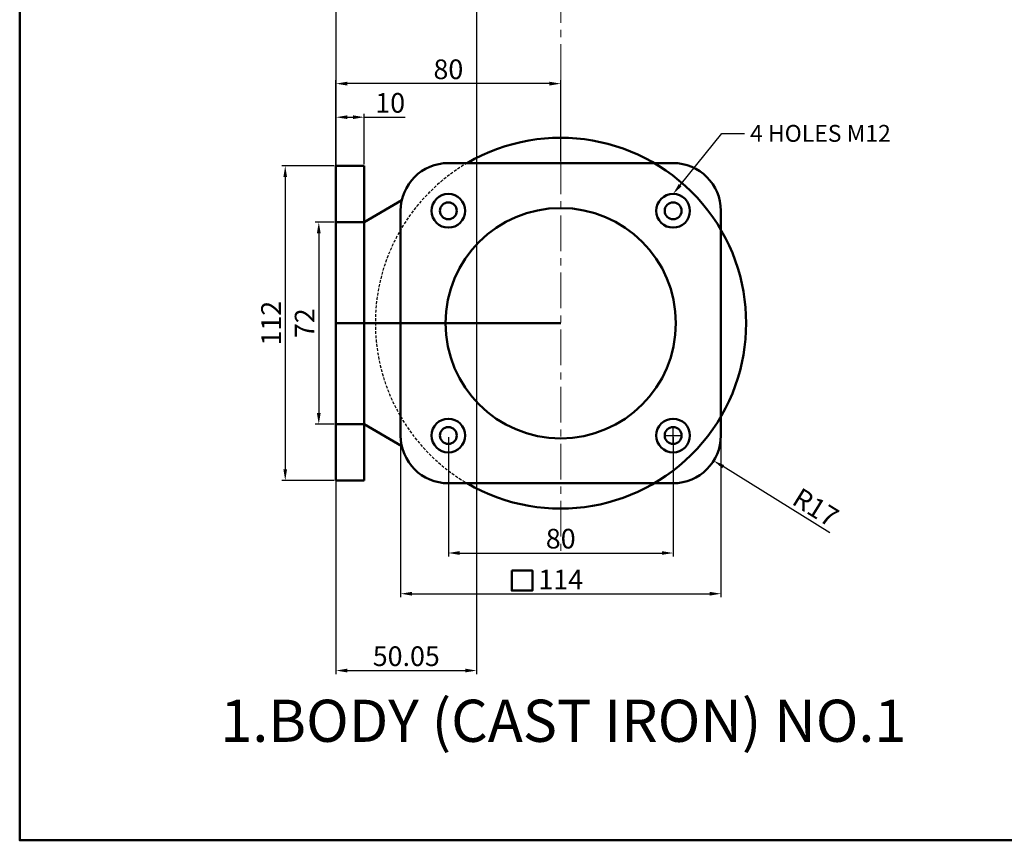
# Model space of a CAD drawing. Units: millimetres. Extents: x 49 to 1001, y -335 to 311.
# Tile 1 of 4: x 49 to 399, y -335 to -43. Entities that reach past the tile are written whole.
import ezdxf
from ezdxf import colors
from ezdxf.entities.mleader import LeaderData, LeaderLine
from ezdxf.math import Vec2, Vec3

# ---------------------------------------------------------------- set-up
doc = ezdxf.new("R2010")
doc.units = ezdxf.units.MM
doc.header["$LTSCALE"] = 0.4
doc.linetypes.add('CENTER', pattern=[50.8, 31.75, -6.35, 6.35, -6.35])
doc.linetypes.add('HIDDEN', pattern=[9.525, 6.35, -3.175])
for name, color, linetype, lineweight in [('M-CNTR', 1, 'CENTER', 18), ('M-DIMS', 2, 'Continuous', 25), ('M-HIDN', 6, 'HIDDEN', 25), ('M-OUTL', 7, 'Continuous', 50), ('M-TEXT', 3, 'Continuous', 25)]:
    doc.layers.add(name, color=color, linetype=linetype, lineweight=lineweight)
doc.styles.get("Standard").update_dxf_attribs({"font": 'arial.ttf'})
doc.dimstyles.new('ISO-25', dxfattribs={"dimtxt": 7, "dimasz": 4, "dimexe": 1.25, "dimexo": 0.625, "dimtad": 1, "dimtxsty": 'Standard', "dimcen": 2.5, "dimadec": 0, "dimazin": 0, "dimtfac": 1, "dimtofl": 0, "dimtmove": 0, "dimatfit": 3, "dimfxl": 1, "dimarcsym": 0})

# ---------------------------------------------------------------- blocks, each defined once
blk = doc.blocks.new('*D17')
at = {"layer": 'Defpoints', "color": 0, "ltscale": 0.4, "transparency": 16777216}
for p in [(171.24, -77.64), (161.24, -94.96), (171.24, -94.96)]:
    blk.add_point(p, dxfattribs=at)
at = {"layer": 'M-DIMS', "color": 0, "lineweight": -2, "ltscale": 0.4, "transparency": 16777216}
for p, q in [((161.24, -94.34), (161.24, -76.39)), ((171.24, -94.34), (171.24, -76.39)), ((165.24, -77.64), (167.24, -77.64)), ((171.24, -77.64), (185.83, -77.64))]:
    blk.add_line(p, q, dxfattribs=at)
at = {"layer": 'M-DIMS', "color": 0, "ltscale": 0.4, "transparency": 16777216}
for points in [[(165.24, -76.97), (165.24, -78.3), (161.24, -77.64)], [(167.24, -76.97), (167.24, -78.3), (171.24, -77.64)]]:
    blk.add_solid(points, dxfattribs=at)
at = {"layer": 'M-DIMS', "color": 0, "ltscale": 0.4, "transparency": 16777216, "insert": (180.53, -73.44), "char_height": 7, "attachment_point": 5}
blk.add_mtext('10', dxfattribs=at)
blk = doc.blocks.new('*D18')
at = {"layer": 'Defpoints', "color": 0, "ltscale": 0.4, "transparency": 16777216}
for p in [(161.24, -94.96), (143.17, -206.96), (161.24, -206.96)]:
    blk.add_point(p, dxfattribs=at)
at = {"layer": 'M-DIMS', "color": 0, "lineweight": -2, "ltscale": 0.4, "transparency": 16777216}
for p, q in [((160.61, -94.96), (141.92, -94.96)), ((143.17, -98.96), (143.17, -202.96)), ((160.61, -206.96), (141.92, -206.96))]:
    blk.add_line(p, q, dxfattribs=at)
at = {"layer": 'M-DIMS', "color": 0, "ltscale": 0.4, "transparency": 16777216}
for points in [[(142.5, -98.96), (143.83, -98.96), (143.17, -94.96)], [(142.5, -202.96), (143.83, -202.96), (143.17, -206.96)]]:
    blk.add_solid(points, dxfattribs=at)
at = {"layer": 'M-DIMS', "color": 0, "ltscale": 0.4, "transparency": 16777216, "insert": (139.03, -150.96), "char_height": 7, "attachment_point": 5, "rotation": 90}
blk.add_mtext('112', dxfattribs=at)
blk = doc.blocks.new('*D19')
at = {"layer": 'Defpoints', "color": 0, "ltscale": 0.4, "transparency": 16777216}
for p in [(161.24, -114.96), (155.12, -186.96), (161.24, -186.96)]:
    blk.add_point(p, dxfattribs=at)
at = {"layer": 'M-DIMS', "color": 0, "lineweight": -2, "ltscale": 0.4, "transparency": 16777216}
for p, q in [((160.61, -114.96), (153.87, -114.96)), ((155.12, -118.96), (155.12, -182.96)), ((160.61, -186.96), (153.87, -186.96))]:
    blk.add_line(p, q, dxfattribs=at)
at = {"layer": 'M-DIMS', "color": 0, "ltscale": 0.4, "transparency": 16777216}
for points in [[(154.45, -118.96), (155.78, -118.96), (155.12, -114.96)], [(154.45, -182.96), (155.78, -182.96), (155.12, -186.96)]]:
    blk.add_solid(points, dxfattribs=at)
at = {"layer": 'M-DIMS', "color": 0, "ltscale": 0.4, "transparency": 16777216, "insert": (150.98, -150.96), "char_height": 7, "attachment_point": 5, "rotation": 90}
blk.add_mtext('72', dxfattribs=at)
blk = doc.blocks.new('*D20')
at = {"layer": 'Defpoints', "color": 0, "ltscale": 0.4, "transparency": 16777216}
for p in [(161.24, -65.69), (241.24, -93.96), (161.24, -114.96)]:
    blk.add_point(p, dxfattribs=at)
at = {"layer": 'M-DIMS', "color": 0, "lineweight": -2, "ltscale": 0.4, "transparency": 16777216}
for p, q in [((161.24, -114.34), (161.24, -64.44)), ((237.24, -65.69), (165.24, -65.69)), ((241.24, -93.34), (241.24, -64.44))]:
    blk.add_line(p, q, dxfattribs=at)
at = {"layer": 'M-DIMS', "color": 0, "ltscale": 0.4, "transparency": 16777216}
for points in [[(165.24, -65.02), (165.24, -66.36), (161.24, -65.69)], [(237.24, -65.02), (237.24, -66.36), (241.24, -65.69)]]:
    blk.add_solid(points, dxfattribs=at)
at = {"layer": 'M-DIMS', "color": 0, "ltscale": 0.4, "transparency": 16777216, "insert": (201.24, -61.49), "char_height": 7, "attachment_point": 5}
blk.add_mtext('80', dxfattribs=at)
blk = doc.blocks.new('*D21')
at = {"layer": 'Defpoints', "color": 0, "ltscale": 0.4, "transparency": 16777216}
for p in [(298.24, -173.69), (184.24, -178.8), (298.24, -247.27)]:
    blk.add_point(p, dxfattribs=at)
at = {"layer": 'M-DIMS', "color": 0, "lineweight": -2, "ltscale": 0.4, "transparency": 16777216}
for p, q in [((298.24, -174.31), (298.24, -248.52)), ((184.24, -179.42), (184.24, -248.52)), ((188.24, -247.27), (294.24, -247.27))]:
    blk.add_line(p, q, dxfattribs=at)
at = {"layer": 'M-DIMS', "color": 0, "ltscale": 0.4, "transparency": 16777216}
for points in [[(188.24, -246.6), (188.24, -247.94), (184.24, -247.27)], [(294.24, -246.6), (294.24, -247.94), (298.24, -247.27)]]:
    blk.add_solid(points, dxfattribs=at)
at = {"layer": 'M-DIMS', "color": 0, "ltscale": 0.4, "transparency": 16777216, "insert": (241.24, -243.13), "char_height": 7, "attachment_point": 5}
blk.add_mtext('114', dxfattribs=at)
blk = doc.blocks.new('*D22')
at = {"layer": 'Defpoints', "color": 0, "ltscale": 0.4, "transparency": 16777216}
for p in [(201.24, -190.96), (281.24, -190.96), (281.24, -232.78)]:
    blk.add_point(p, dxfattribs=at)
at = {"layer": 'M-DIMS', "color": 0, "lineweight": -2, "ltscale": 0.4, "transparency": 16777216}
for p, q in [((201.24, -191.59), (201.24, -234.03)), ((281.24, -191.59), (281.24, -234.03)), ((205.24, -232.78), (277.24, -232.78))]:
    blk.add_line(p, q, dxfattribs=at)
at = {"layer": 'M-DIMS', "color": 0, "ltscale": 0.4, "transparency": 16777216}
for points in [[(205.24, -232.11), (205.24, -233.44), (201.24, -232.78)], [(277.24, -232.11), (277.24, -233.44), (281.24, -232.78)]]:
    blk.add_solid(points, dxfattribs=at)
at = {"layer": 'M-DIMS', "color": 0, "ltscale": 0.4, "transparency": 16777216, "insert": (241.24, -228.58), "char_height": 7, "attachment_point": 5}
blk.add_mtext('80', dxfattribs=at)
blk = doc.blocks.new('*D23')
at = {"layer": 'Defpoints', "color": 0, "ltscale": 0.4, "transparency": 16777216}
for p in [(281.24, -190.96), (295.68, -199.93)]:
    blk.add_point(p, dxfattribs=at)
at = {"layer": 'M-DIMS', "color": 0, "lineweight": -2, "ltscale": 0.4, "transparency": 16777216}
for p, q in [((281.24, -193.46), (281.24, -188.46)), ((278.74, -190.96), (283.74, -190.96)), ((336.99, -225.58), (299.08, -202.04))]:
    blk.add_line(p, q, dxfattribs=at)
at = {"layer": 'M-DIMS', "color": 0, "ltscale": 0.4, "transparency": 16777216}
blk.add_solid([(299.43, -201.47), (298.73, -202.61), (295.68, -199.93)], dxfattribs=at)
at = {"layer": 'M-DIMS', "color": 0, "ltscale": 0.4, "transparency": 16777216, "insert": (331.53, -217.32), "char_height": 7, "attachment_point": 5, "rotation": 328.1606}
blk.add_mtext('R17', dxfattribs=at)
blk = doc.blocks.new('BOLT-HOLE-12')
at = {"ltscale": 0.4}
for radius in [6, 3]:
    blk.add_circle((6, 6), radius, dxfattribs=at)
blk = doc.blocks.new('*D58')
at = {"layer": 'Defpoints', "color": 0, "ltscale": 0.4, "transparency": 16777216}
for p in [(211.28, 81.71), (161.24, 58.7), (211.28, -274.62)]:
    blk.add_point(p, dxfattribs=at)
at = {"layer": 'M-DIMS', "color": 0, "lineweight": -2, "ltscale": 0.4, "transparency": 16777216}
for p, q in [((211.28, 81.09), (211.28, -275.87)), ((161.24, 58.08), (161.24, -275.87)), ((165.24, -274.62), (207.28, -274.62))]:
    blk.add_line(p, q, dxfattribs=at)
at = {"layer": 'M-DIMS', "color": 0, "ltscale": 0.4, "transparency": 16777216}
for points in [[(165.24, -273.95), (165.24, -275.28), (161.24, -274.62)], [(207.28, -273.95), (207.28, -275.28), (211.28, -274.62)]]:
    blk.add_solid(points, dxfattribs=at)
at = {"layer": 'M-DIMS', "color": 0, "ltscale": 0.4, "transparency": 16777216, "insert": (186.26, -270.42), "char_height": 7, "attachment_point": 5}
blk.add_mtext('50.05', dxfattribs=at)

msp = doc.modelspace()

# ---------------------------------------------------------------- linework, layer by layer
at = {"layer": 'M-CNTR'}
msp.add_line((241.2373, 232.8267), (241.2373, -233.1822), dxfattribs=at)
at = {"layer": 'M-HIDN', "ltscale": 0.4}
msp.add_arc((241.2373, -150.9613), 66, 120.272641, 239.727359, dxfattribs=at)
at = {"layer": 'M-OUTL', "ltscale": 0.4}
for p, q in [((161.2373, -150.9613), (161.2373, -94.9613)), ((161.2373, -94.9613), (171.2373, -94.9613)), ((171.2373, -94.9613), (171.2373, -206.9613)), ((171.2373, -114.9613), (184.6554, -107.2144)), ((171.2373, -114.9613), (161.2373, -114.9613)), ((241.2373, -150.9613), (161.2373, -150.9613)), ((161.2373, -206.9613), (161.2373, -150.9613)), ((171.2373, -186.9613), (161.2373, -186.9613)), ((171.2373, -186.9613), (184.6554, -194.7082)), ((171.2373, -206.9613), (161.2373, -206.9613))]:
    msp.add_line(p, q, dxfattribs=at)
for points in [[(48.6466, 311.3462), (1001.3348, 311.3462), (1001.3348, -335.0483), (48.6466, -335.0483)], [(223.8267, -239.0323), (231.1417, -239.0323), (231.1417, -246.1666), (223.8267, -246.1666)]]:
    msp.add_lwpolyline(points, close=True, dxfattribs=at)
msp.add_lwpolyline([(201.2373, -93.9613), (281.2373, -93.9613, -0.41421356), (298.2373, -110.9613), (298.2373, -190.9613, -0.41421356), (281.2373, -207.9613), (201.2373, -207.9613, -0.41421356), (184.2373, -190.9613), (184.2373, -110.9613, -0.41421356)], format="xyb", close=True, dxfattribs=at)
msp.add_circle((241.2373, -150.9613), 41, dxfattribs=at)
msp.add_arc((241.2373, -150.9613), 66, 239.727359, 120.272641, dxfattribs=at)

# ---------------------------------------------------------------- block references
at = {"layer": 'M-OUTL'}
for p in [(195.237, -116.961), (275.237, -116.961), (195.237, -196.961), (275.237, -196.961)]:
    msp.add_blockref('BOLT-HOLE-12', p, dxfattribs=at)

# ---------------------------------------------------------------- texts
at = {"layer": 'M-TEXT', "ltscale": 0.4, "insert": (120.105, -284.9979), "char_height": 15, "attachment_point": 1}
msp.add_mtext_dynamic_manual_height_columns('1.BODY (CAST IRON) NO.1', width=263.462389, gutter_width=12.5, heights=[0], dxfattribs=at)

# ---------------------------------------------------------------- dimensions: what is measured, and where the dimension line sits
at = {"layer": 'M-DIMS', "ltscale": 0.4}
for base, p1, p2, override, picture, middle in [((211.2829, -274.6166), (161.2373, 58.7021), (211.2829, 81.7143), {"dimdec": 2, "dimlfac": 1, "dimrnd": 0, "dimzin": 0, "dimdsep": 46, "dimlunit": 2}, '*D58', (186.2601, -270.4176)), ((161.2373, -65.6885), (241.2373, -93.9613), (161.2373, -114.9613), {"dimclrd": 0, "dimclre": 0, "dimclrt": 0}, '*D20', (201.2373, -61.4895)), ((171.2373, -77.6381), (161.2373, -94.9613), (171.2373, -94.9613), {"dimclrd": 0, "dimclre": 0, "dimclrt": 0}, '*D17', (180.5346, -73.439)), ((298.2373, -247.2713), (184.2373, -178.7991), (298.2373, -173.6859), {"dimclrd": 0, "dimclre": 0, "dimclrt": 0}, '*D21', (241.2373, -243.132)), ((281.2373, -232.777), (201.2373, -190.9613), (281.2373, -190.9613), {"dimclrd": 0, "dimclre": 0, "dimclrt": 0}, '*D22', (241.2373, -228.5779))]:
    dim = msp.add_linear_dim(base=base, p1=p1, p2=p2, dimstyle='ISO-25', override=override, dxfattribs=at)
    dim.commit()
    dim.dimension.update_dxf_attribs({"geometry": picture, "text_midpoint": middle})
for base, p1, p2, picture, middle in [((143.1676, -206.9613), (161.2373, -94.9613), (161.2373, -206.9613), '*D18', (139.0282, -150.9613)), ((155.1167, -186.9613), (161.2373, -114.9613), (161.2373, -186.9613), '*D19', (150.9774, -150.9613))]:
    dim = msp.add_linear_dim(base=base, p1=p1, p2=p2, angle=90, dimstyle='ISO-25', override={"dimclrd": 0, "dimclre": 0, "dimclrt": 0}, dxfattribs=at)
    dim.commit()
    dim.dimension.update_dxf_attribs({"geometry": picture, "text_midpoint": middle})
dim = msp.add_radius_dim(center=(281.2373, -190.9613), mpoint=(295.6793, -199.9295), dimstyle='ISO-25', override={"dimclrd": 0, "dimclre": 0, "dimclrt": 0}, dxfattribs=at)
dim.commit()
dim.dimension.update_dxf_attribs({"geometry": '*D23', "text_midpoint": (329.351, -220.8389), "dimtype": 164})

# ---------------------------------------------------------------- leaders
ml = msp.add_multileader_mtext('Standard', dxfattribs=at)
ml.set_content('4 HOLES M12', color=256)
ml.set_leader_properties()
ml.build(insert=Vec2(0, 0))
ctx = ml.context
ctx.base_point, ctx.char_height, ctx.plane_origin = Vec3(306.621, -83.4432), 6, Vec3(281.2373, -104.9613)
notes = []
notes.append((ctx, [(0, (1, 1, 0), (298.621, -83.4432), (1, 0), 8, [(0, [(281.2373, -104.9613)], 0, [])])]))
ctx.mtext.insert, ctx.mtext.flow_direction = Vec3(308.621, -80.3921), 5
for ctx, leaders in notes:
    for number, flags, end, landing, length, lines in leaders:
        leader = LeaderData()
        leader.index, (leader.has_last_leader_line, leader.has_dogleg_vector, leader.attachment_direction) = number, flags
        leader.last_leader_point, leader.dogleg_vector, leader.dogleg_length = Vec3(end), Vec3(landing), length
        for number, points, colour, breaks in lines:
            line = LeaderLine()
            line.index, line.vertices, line.color, line.breaks = number, Vec3.list(points), colors.encode_raw_color(colour), breaks
            leader.lines.append(line)
        ctx.leaders.append(leader)

doc.saveas('drawing.dxf')
